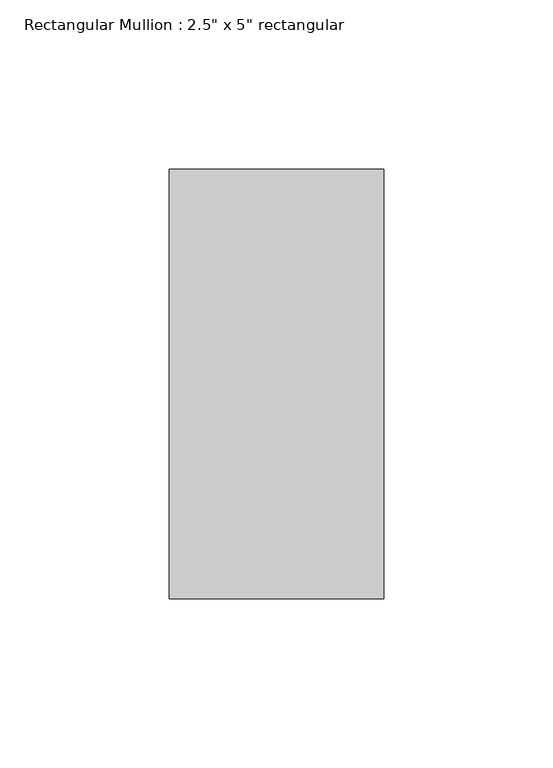
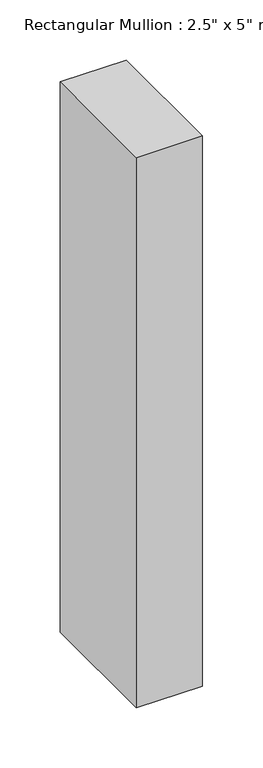
"""IFC4 building model written with IfcOpenShell, lengths in millimetres: member geometry."""

from ifc_helpers import new_model, si_unit, frame, origin, place, context, project, spatial, polyline, outline, extrude, source, transform, mapped, element, save


def member_50cacee6(model_context):
    return source(origin(), model_context, "Body", "SweptSolid", [
        extrude(outline(polyline([(0.0, 63.5), (0.0, -63.5), (-63.5, -63.5), (-63.5, 63.5), (0.0, 63.5)])), frame((0.0, 0.0, -558.8), z_axis=(0.0, 0.0, 1.0), x_axis=(1.0, 0.0, 0.0)), (0.0, 0.0, 1.0), 558.8),
    ])


if __name__ == "__main__":
    model = new_model("IFC4")
    model_context = context("Model", 3, world=origin())
    ifc_project = project(units=[si_unit("LENGTHUNIT", "METRE", prefix="MILLI")], contexts=[model_context])
    site = spatial("IfcSite", under=ifc_project)
    building = spatial("IfcBuilding", under=site)
    placement = place(None, origin())
    member_shape = member_50cacee6(model_context)
    element("IfcMember", 1, ObjectType="Rectangular Mullion : 2.5\" x 5\" rectangular", at=placement, inside=building, context=model_context, shape_type="MappedRepresentation", body=[
        mapped(member_shape, transform((0.0, 0.0, 0.0), x_axis=(1.0, 0.0, 0.0), y_axis=(0.0, 1.0, 0.0), z_axis=(0.0, 0.0, 1.0))),
    ])
    save(model, "model.ifc")

# Revit data of these elements
# Type "Rectangular Mullion : 2.5\" x 5\" rectangular"
#   built-in parameter 1007304 = 0.416667 (stored number, unit not read)
#   built-in parameter 1007301 = 0.104167 (stored number, unit not read)
#   built-in parameter 1007300 = 0.104167 (stored number, unit not read)
